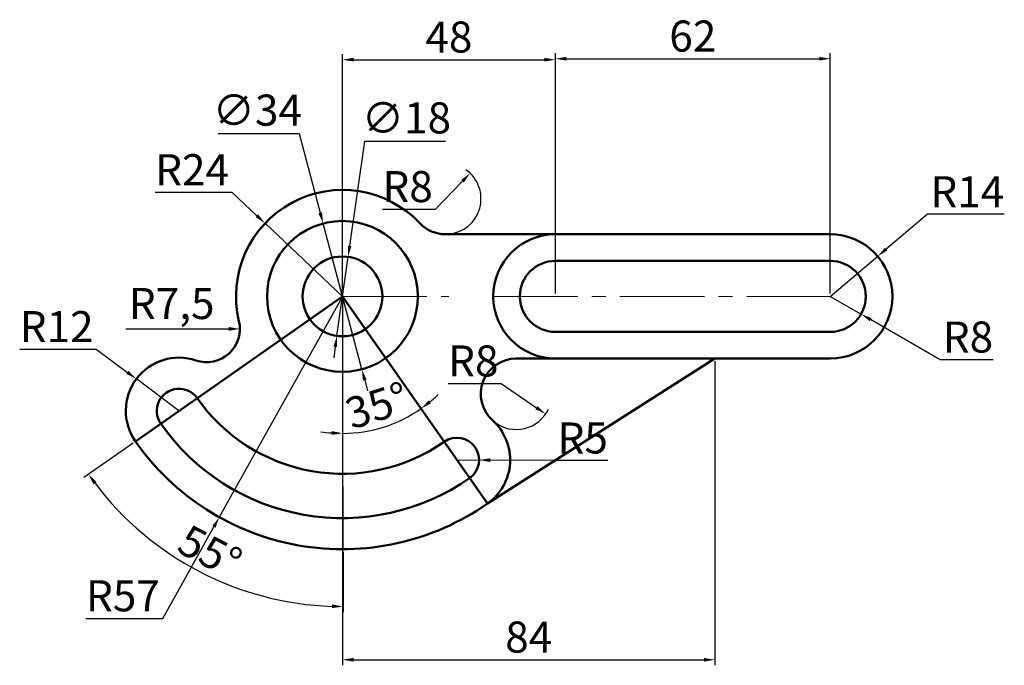
# Model space of a CAD drawing. Units: millimetres. Extents: x -3 to 219, y 128 to 273.
import ezdxf

# ---------------------------------------------------------------- set-up
doc = ezdxf.new("R2010")
doc.units = ezdxf.units.MM
doc.linetypes.add('CENTER2', pattern=[28.575, 19.05, -3.175, 3.175, -3.175])
for name, color, linetype, lineweight in [('M-CNTR', 4, 'CENTER2', 18), ('M-CONS', 8, 'Continuous', 13), ('M-DIMS', 2, 'Continuous', 25), ('M-OUTL', 7, 'Continuous', 50)]:
    doc.layers.add(name, color=color, linetype=linetype, lineweight=lineweight)
doc.styles.get("Standard").update_dxf_attribs({"font": 'arial.ttf'})
doc.dimstyles.new('ISO-25', dxfattribs={"dimtxt": 7, "dimasz": 2.5, "dimexe": 1.25, "dimexo": 0.625, "dimtad": 1, "dimtoh": 1, "dimdec": 1, "dimtxsty": 'Standard', "dimcen": 2.5, "dimadec": 0, "dimazin": 0, "dimtfac": 1, "dimtdec": 1, "dimtmove": 0, "dimatfit": 3, "dimfxl": 1, "dimarcsym": 0})

# ---------------------------------------------------------------- blocks, each defined once
blk = doc.blocks.new('*D1')
at = {"layer": 'Defpoints', "color": 0, "transparency": 16777216}
for p in [(118, 264.15), (70, 210.79), (118, 210.79)]:
    blk.add_point(p, dxfattribs=at)
at = {"layer": 'M-DIMS', "color": 0, "lineweight": -2, "transparency": 16777216}
for p, q in [((70, 211.42), (70, 265.4)), ((118, 211.42), (118, 265.4)), ((72.5, 264.15), (115.5, 264.15))]:
    blk.add_line(p, q, dxfattribs=at)
at = {"layer": 'M-DIMS', "color": 0, "transparency": 16777216}
for points in [[(72.5, 264.57), (72.5, 263.74), (70, 264.15)], [(115.5, 264.57), (115.5, 263.74), (118, 264.15)]]:
    blk.add_solid(points, dxfattribs=at)
at = {"layer": 'M-DIMS', "color": 0, "transparency": 16777216, "insert": (94, 268.35), "char_height": 7, "attachment_point": 5}
blk.add_mtext('48', dxfattribs=at)
blk = doc.blocks.new('*D2')
at = {"layer": 'Defpoints', "color": 0, "transparency": 16777216}
for p in [(180, 264.37), (118, 210.79), (180, 210.79)]:
    blk.add_point(p, dxfattribs=at)
at = {"layer": 'M-DIMS', "color": 0, "lineweight": -2, "transparency": 16777216}
for p, q in [((118, 211.42), (118, 265.62)), ((120.5, 264.37), (177.5, 264.37)), ((180, 211.42), (180, 265.62))]:
    blk.add_line(p, q, dxfattribs=at)
at = {"layer": 'M-DIMS', "color": 0, "transparency": 16777216}
for points in [[(120.5, 264.79), (120.5, 263.95), (118, 264.37)], [(177.5, 264.79), (177.5, 263.95), (180, 264.37)]]:
    blk.add_solid(points, dxfattribs=at)
at = {"layer": 'M-DIMS', "color": 0, "transparency": 16777216, "insert": (149, 268.57), "char_height": 7, "attachment_point": 5}
blk.add_mtext('62', dxfattribs=at)
blk = doc.blocks.new('*D3')
at = {"layer": 'Defpoints', "color": 0, "transparency": 16777216}
for p in [(70, 210.79), (154, 196.79), (154, 128.88)]:
    blk.add_point(p, dxfattribs=at)
at = {"layer": 'M-DIMS', "color": 0, "lineweight": -2, "transparency": 16777216}
for p, q in [((70, 210.17), (70, 127.63)), ((154, 196.17), (154, 127.63)), ((72.5, 128.88), (151.5, 128.88))]:
    blk.add_line(p, q, dxfattribs=at)
at = {"layer": 'M-DIMS', "color": 0, "transparency": 16777216}
for points in [[(72.5, 129.29), (72.5, 128.46), (70, 128.88)], [(151.5, 129.29), (151.5, 128.46), (154, 128.88)]]:
    blk.add_solid(points, dxfattribs=at)
at = {"layer": 'M-DIMS', "color": 0, "transparency": 16777216, "insert": (112, 133.08), "char_height": 7, "attachment_point": 5}
blk.add_mtext('84', dxfattribs=at)
blk = doc.blocks.new('*D4')
at = {"layer": 'Defpoints', "color": 0, "transparency": 16777216}
for p in [(190.69, 219.84), (180, 210.79)]:
    blk.add_point(p, dxfattribs=at)
at = {"layer": 'M-DIMS', "color": 0, "lineweight": -2, "transparency": 16777216}
for p, q in [((201.91, 229.34), (192.59, 221.46)), ((219.24, 229.34), (201.91, 229.34)), ((180, 210.79), (190.69, 219.84))]:
    blk.add_line(p, q, dxfattribs=at)
at = {"layer": 'M-DIMS', "color": 0, "transparency": 16777216}
blk.add_solid([(192.33, 221.77), (192.86, 221.14), (190.69, 219.84)], dxfattribs=at)
at = {"layer": 'M-DIMS', "color": 0, "transparency": 16777216, "insert": (210.89, 233.48), "char_height": 7, "attachment_point": 5}
blk.add_mtext('R14', dxfattribs=at)
blk = doc.blocks.new('*D5')
at = {"layer": 'Defpoints', "color": 0, "transparency": 16777216}
for p in [(180, 210.79), (186.93, 206.8)]:
    blk.add_point(p, dxfattribs=at)
at = {"layer": 'M-DIMS', "color": 0, "lineweight": -2, "transparency": 16777216}
for p, q in [((180, 210.79), (186.93, 206.8)), ((204.76, 196.52), (189.1, 205.55)), ((216.69, 196.52), (204.76, 196.52))]:
    blk.add_line(p, q, dxfattribs=at)
at = {"layer": 'M-DIMS', "color": 0, "transparency": 16777216}
blk.add_solid([(189.31, 205.91), (188.89, 205.19), (186.93, 206.8)], dxfattribs=at)
at = {"layer": 'M-DIMS', "color": 0, "transparency": 16777216, "insert": (211.04, 200.72), "char_height": 7, "attachment_point": 5}
blk.add_mtext('R8', dxfattribs=at)
blk = doc.blocks.new('*D6')
at = {"layer": 'Defpoints', "color": 0, "transparency": 16777216}
for p in [(98.79, 238.55), (93.24, 232.79)]:
    blk.add_point(p, dxfattribs=at)
at = {"layer": 'M-DIMS', "color": 0, "lineweight": -2, "transparency": 16777216}
for p, q in [((90.97, 230.44), (97.06, 236.75)), ((79.04, 230.44), (90.97, 230.44))]:
    blk.add_line(p, q, dxfattribs=at)
blk.add_arc((93.24, 232.79), 8, 274.4762, 54.9956, dxfattribs=at)
at = {"layer": 'M-DIMS', "color": 0, "transparency": 16777216}
blk.add_solid([(96.76, 237.04), (97.36, 236.46), (98.79, 238.55)], dxfattribs=at)
at = {"layer": 'M-DIMS', "color": 0, "transparency": 16777216, "insert": (84.69, 234.63), "char_height": 7, "attachment_point": 5}
blk.add_mtext('R8', dxfattribs=at)
blk = doc.blocks.new('*D7')
at = {"layer": 'Defpoints', "color": 0, "transparency": 16777216}
for p in [(70, 210.79), (70, 210.79), (76.29, 180.55), (102.7, 164.1), (70.13, 153.79)]:
    blk.add_point(p, dxfattribs=at)
at = {"layer": 'M-DIMS', "color": 0, "lineweight": -2, "transparency": 16777216}
for start, end in [(309.6386, 314.2772), (270.1287, 305), (260.8515, 265.4901)]:
    blk.add_arc((70, 210.79), 30.89, start, end, dxfattribs=at)
at = {"layer": 'M-DIMS', "color": 0, "transparency": 16777216}
for points in [[(89.96, 186.68), (89.45, 187.34), (87.72, 185.49)], [(67.59, 180.42), (67.56, 179.58), (70.07, 179.91)]]:
    blk.add_solid(points, dxfattribs=at)
at = {"layer": 'M-DIMS', "color": 0, "transparency": 16777216, "insert": (78.05, 185.35), "char_height": 7, "attachment_point": 5, "rotation": 17.5643}
blk.add_mtext('35°', dxfattribs=at)
blk = doc.blocks.new('*D8')
at = {"layer": 'Defpoints', "color": 0, "transparency": 16777216}
for p in [(70, 210.79), (70, 210.79), (23.31, 178.1), (28.3, 154.69), (70.13, 153.79)]:
    blk.add_point(p, dxfattribs=at)
at = {"layer": 'M-DIMS', "color": 0, "lineweight": -2, "transparency": 16777216}
for p, q in [((22.8, 177.74), (11.71, 169.98)), ((70.13, 153.17), (70.16, 139.64))]:
    blk.add_line(p, q, dxfattribs=at)
blk.add_arc((70, 210.79), 69.91, 217.0492, 268.0795, dxfattribs=at)
at = {"layer": 'M-DIMS', "color": 0, "transparency": 16777216}
for points in [[(13.87, 168.43), (14.55, 168.92), (12.74, 170.7)], [(67.67, 141.34), (67.65, 140.51), (70.16, 140.89)]]:
    blk.add_solid(points, dxfattribs=at)
at = {"layer": 'M-DIMS', "color": 0, "transparency": 16777216, "insert": (39.72, 152.47), "char_height": 7, "attachment_point": 5, "rotation": 332.5643}
blk.add_mtext('55°', dxfattribs=at)
blk = doc.blocks.new('*D9')
at = {"layer": 'Defpoints', "color": 0, "transparency": 16777216}
for p in [(70, 210.79), (42.23, 161.02)]:
    blk.add_point(p, dxfattribs=at)
at = {"layer": 'M-DIMS', "color": 0, "lineweight": -2, "transparency": 16777216}
for p, q in [((70, 210.79), (42.23, 161.02)), ((29.49, 138.2), (41.01, 158.84)), ((12.14, 138.2), (29.49, 138.2))]:
    blk.add_line(p, q, dxfattribs=at)
at = {"layer": 'M-DIMS', "color": 0, "transparency": 16777216}
blk.add_solid([(40.64, 159.04), (41.37, 158.63), (42.23, 161.02)], dxfattribs=at)
at = {"layer": 'M-DIMS', "color": 0, "transparency": 16777216, "insert": (20.5, 142.39), "char_height": 7, "attachment_point": 5}
blk.add_mtext('R57', dxfattribs=at)
blk = doc.blocks.new('*D10')
at = {"layer": 'Defpoints', "color": 0, "transparency": 16777216}
for p in [(109.2, 188.79), (115.81, 184.29)]:
    blk.add_point(p, dxfattribs=at)
at = {"layer": 'M-DIMS', "color": 0, "lineweight": -2, "transparency": 16777216}
for p, q in [((93.84, 191.13), (105.77, 191.13)), ((105.77, 191.13), (113.74, 185.7))]:
    blk.add_line(p, q, dxfattribs=at)
blk.add_arc((109.2, 188.79), 8, 232.4717, 334.6668, dxfattribs=at)
at = {"layer": 'M-DIMS', "color": 0, "transparency": 16777216}
blk.add_solid([(113.98, 186.04), (113.51, 185.35), (115.81, 184.29)], dxfattribs=at)
at = {"layer": 'M-DIMS', "color": 0, "transparency": 16777216, "insert": (99.49, 195.33), "char_height": 7, "attachment_point": 5}
blk.add_mtext('R8', dxfattribs=at)
blk = doc.blocks.new('*D11')
at = {"layer": 'Defpoints', "color": 0, "transparency": 16777216}
for p in [(39.37, 203.46), (46.87, 203.46)]:
    blk.add_point(p, dxfattribs=at)
at = {"layer": 'M-DIMS', "color": 0, "lineweight": -2, "transparency": 16777216}
blk.add_line((21.12, 203.46), (44.37, 203.46), dxfattribs=at)
at = {"layer": 'M-DIMS', "color": 0, "transparency": 16777216}
blk.add_solid([(44.37, 203.88), (44.37, 203.05), (46.87, 203.46)], dxfattribs=at)
at = {"layer": 'M-DIMS', "color": 0, "transparency": 16777216, "insert": (31.49, 208.28), "char_height": 7, "attachment_point": 5}
blk.add_mtext('R7,5', dxfattribs=at)
blk = doc.blocks.new('*D12')
at = {"layer": 'Defpoints', "color": 0, "transparency": 16777216}
for p in [(52.54, 227.26), (70, 210.79)]:
    blk.add_point(p, dxfattribs=at)
at = {"layer": 'M-DIMS', "color": 0, "lineweight": -2, "transparency": 16777216}
for p, q in [((27.74, 234.3), (45.06, 234.3)), ((45.06, 234.3), (50.72, 228.97)), ((70, 210.79), (52.54, 227.26))]:
    blk.add_line(p, q, dxfattribs=at)
at = {"layer": 'M-DIMS', "color": 0, "transparency": 16777216}
blk.add_solid([(51, 229.27), (50.43, 228.67), (52.54, 227.26)], dxfattribs=at)
at = {"layer": 'M-DIMS', "color": 0, "transparency": 16777216, "insert": (36.09, 238.44), "char_height": 7, "attachment_point": 5}
blk.add_mtext('R24', dxfattribs=at)
blk = doc.blocks.new('*D13')
at = {"layer": 'Defpoints', "color": 0, "transparency": 16777216}
for p in [(71.27, 219.7), (68.74, 201.88)]:
    blk.add_point(p, dxfattribs=at)
at = {"layer": 'M-DIMS', "color": 0, "lineweight": -2, "transparency": 16777216}
for p, q in [((74.96, 245.72), (71.62, 222.18)), ((93.25, 245.72), (74.96, 245.72)), ((68.74, 201.88), (71.27, 219.7)), ((68.38, 199.41), (68.03, 196.93))]:
    blk.add_line(p, q, dxfattribs=at)
at = {"layer": 'M-DIMS', "color": 0, "transparency": 16777216}
for points in [[(71.21, 222.24), (72.03, 222.12), (71.27, 219.7)], [(67.97, 199.47), (68.8, 199.35), (68.74, 201.88)]]:
    blk.add_solid(points, dxfattribs=at)
at = {"layer": 'M-DIMS', "color": 0, "transparency": 16777216, "insert": (84.42, 250.12), "char_height": 7, "attachment_point": 5}
blk.add_mtext('∅18', dxfattribs=at)
blk = doc.blocks.new('*D14')
at = {"layer": 'Defpoints', "color": 0, "transparency": 16777216}
for p in [(65.63, 227.22), (74.38, 194.37)]:
    blk.add_point(p, dxfattribs=at)
at = {"layer": 'M-DIMS', "color": 0, "lineweight": -2, "transparency": 16777216}
for p, q in [((41.99, 247.48), (60.23, 247.48)), ((60.23, 247.48), (64.98, 229.64)), ((74.38, 194.37), (65.63, 227.22)), ((75.02, 191.95), (75.66, 189.53))]:
    blk.add_line(p, q, dxfattribs=at)
at = {"layer": 'M-DIMS', "color": 0, "transparency": 16777216}
for points in [[(65.39, 229.74), (64.58, 229.53), (65.63, 227.22)], [(75.42, 192.06), (74.62, 191.84), (74.38, 194.37)]]:
    blk.add_solid(points, dxfattribs=at)
at = {"layer": 'M-DIMS', "color": 0, "transparency": 16777216, "insert": (50.8, 251.87), "char_height": 7, "attachment_point": 5}
blk.add_mtext('∅34', dxfattribs=at)
blk = doc.blocks.new('*D15')
at = {"layer": 'Defpoints', "color": 0, "transparency": 16777216}
for p in [(23.53, 192.17), (33.14, 184.98)]:
    blk.add_point(p, dxfattribs=at)
at = {"layer": 'M-DIMS', "color": 0, "lineweight": -2, "transparency": 16777216}
for p, q in [((-2.78, 198.93), (14.5, 198.93)), ((14.5, 198.93), (21.53, 193.67)), ((33.14, 184.98), (23.53, 192.17))]:
    blk.add_line(p, q, dxfattribs=at)
at = {"layer": 'M-DIMS', "color": 0, "transparency": 16777216}
blk.add_solid([(21.78, 194), (21.28, 193.34), (23.53, 192.17)], dxfattribs=at)
at = {"layer": 'M-DIMS', "color": 0, "transparency": 16777216, "insert": (5.55, 203.07), "char_height": 7, "attachment_point": 5}
blk.add_mtext('R12', dxfattribs=at)
blk = doc.blocks.new('*D16')
at = {"layer": 'Defpoints', "color": 0, "transparency": 16777216}
for p in [(95.81, 173.93), (100.81, 173.9)]:
    blk.add_point(p, dxfattribs=at)
at = {"layer": 'M-DIMS', "color": 0, "lineweight": -2, "transparency": 16777216}
for p, q in [((95.81, 173.93), (100.81, 173.9)), ((117.87, 173.77), (103.31, 173.88)), ((129.84, 173.77), (117.87, 173.77))]:
    blk.add_line(p, q, dxfattribs=at)
at = {"layer": 'M-DIMS', "color": 0, "transparency": 16777216}
blk.add_solid([(103.32, 174.29), (103.31, 173.46), (100.81, 173.9)], dxfattribs=at)
at = {"layer": 'M-DIMS', "color": 0, "transparency": 16777216, "insert": (124.17, 177.96), "char_height": 7, "attachment_point": 5}
blk.add_mtext('R5', dxfattribs=at)

msp = doc.modelspace()

# ---------------------------------------------------------------- linework, layer by layer
at = {"layer": 'M-CNTR'}
for p, q in [((70, 153.79), (70, 234.79)), ((70, 210.79), (94, 210.79)), ((104, 210.79), (180, 210.79))]:
    msp.add_line(p, q, dxfattribs=at)
at = {"layer": 'M-CONS'}
for p, q in [((70, 210.79), (70.13, 153.79)), ((104, 196.79), (104, 196.75))]:
    msp.add_line(p, q, dxfattribs=at)
at = {"layer": 'M-OUTL'}
msp.add_lwpolyline([(154, 196.79), (102.7, 164.1, 0.482318), (103.84, 182.85, -0.687252), (109.2, 196.79), (118, 196.79), (180, 196.79, 1), (180, 224.79), (93.24, 224.79, -0.206032), (87.43, 227.29, 0.767514), (46.66, 205.21, -0.589528), (36.97, 196.35, 0.72403), (23.31, 178.1), (70, 210.79), (102.7, 164.1, -0.414214), (23.31, 178.1)], format="xyb", dxfattribs=at)
for points in [[(118, 202.79), (180, 202.79, 1), (180, 218.79), (118, 218.79, 1)], [(98.68, 169.84, 1), (92.94, 178.03, -0.414214), (37.24, 187.85, 1), (29.04, 182.12, 0.414214)]]:
    msp.add_lwpolyline(points, format="xyb", close=True, dxfattribs=at)
for radius in [17, 9]:
    msp.add_circle((70, 210.79), radius, dxfattribs=at)
msp.add_arc((118, 210.79), 14, 90, 270, dxfattribs=at)

# ---------------------------------------------------------------- dimensions: what is measured, and where the dimension line sits
at = {"layer": 'M-DIMS'}
for base, p1, p2, picture, middle in [((180, 264.37), (118, 210.79), (180, 210.79), '*D2', (149, 268.57)), ((154, 128.88), (70, 210.79), (154, 196.79), '*D3', (112, 133.08))]:
    dim = msp.add_linear_dim(base=base, p1=p1, p2=p2, dimstyle='ISO-25', override={"dimclrd": 0, "dimclre": 0, "dimclrt": 0}, dxfattribs=at)
    dim.commit()
    dim.dimension.update_dxf_attribs({"geometry": picture, "text_midpoint": middle})
dim = msp.add_aligned_dim(p1=(70, 210.79), p2=(118, 210.79), distance=53.36, dimstyle='ISO-25', override={"dimclrd": 0, "dimclre": 0, "dimclrt": 0}, dxfattribs=at)
dim.commit()
dim.dimension.update_dxf_attribs({"geometry": '*D1', "text_midpoint": (94, 268.35)})
for p1, p2, picture, middle in [((74.38, 194.37), (65.63, 227.22), '*D14', (50.8, 247.48)), ((68.74, 201.88), (71.27, 219.7), '*D13', (84.42, 245.72))]:
    dim = msp.add_diameter_dim_2p(p1=p1, p2=p2, dimstyle='ISO-25', override={"dimclrd": 0, "dimclre": 0, "dimclrt": 0}, dxfattribs=at)
    dim.commit()
    dim.dimension.update_dxf_attribs({"geometry": picture, "text_midpoint": middle, "dimtype": 163})
for center, mpoint, picture, middle in [((70, 210.79), (52.54, 227.26), '*D12', (36.09, 234.3)), ((93.24, 232.79), (98.79, 238.55), '*D6', (84.69, 230.44)), ((180, 210.79), (190.69, 219.84), '*D4', (210.89, 229.34)), ((39.37, 203.46), (46.87, 203.46), '*D11', (31.49, 203.46)), ((70, 210.79), (42.23, 161.02), '*D9', (20.5, 138.2)), ((180, 210.79), (186.93, 206.8), '*D5', (211.04, 196.52)), ((33.14, 184.98), (23.53, 192.17), '*D15', (5.55, 198.93)), ((109.2, 188.79), (115.81, 184.29), '*D10', (99.49, 191.13)), ((95.81, 173.93), (100.81, 173.9), '*D16', (117.87, 173.77))]:
    dim = msp.add_radius_dim(center=center, mpoint=mpoint, dimstyle='ISO-25', override={"dimclrd": 0, "dimclre": 0, "dimclrt": 0}, dxfattribs=at)
    dim.commit()
    dim.dimension.update_dxf_attribs({"geometry": picture, "text_midpoint": middle, "dimtype": 164})
for base, line1, picture, middle in [((28.3, 154.69), ((23.31, 178.1), (70, 210.79)), '*D8', (39.72, 152.47)), ((76.29, 180.55), ((70, 210.79), (102.7, 164.1)), '*D7', (78.05, 185.35))]:
    dim = msp.add_angular_dim_2l(base=base, line1=line1, line2=((70, 210.79), (70.13, 153.79)), dimstyle='ISO-25', override={"dimclrd": 0, "dimclre": 0, "dimclrt": 0}, dxfattribs=at)
    dim.commit()
    dim.dimension.update_dxf_attribs({"geometry": picture, "text_midpoint": middle})

doc.saveas('drawing.dxf')
